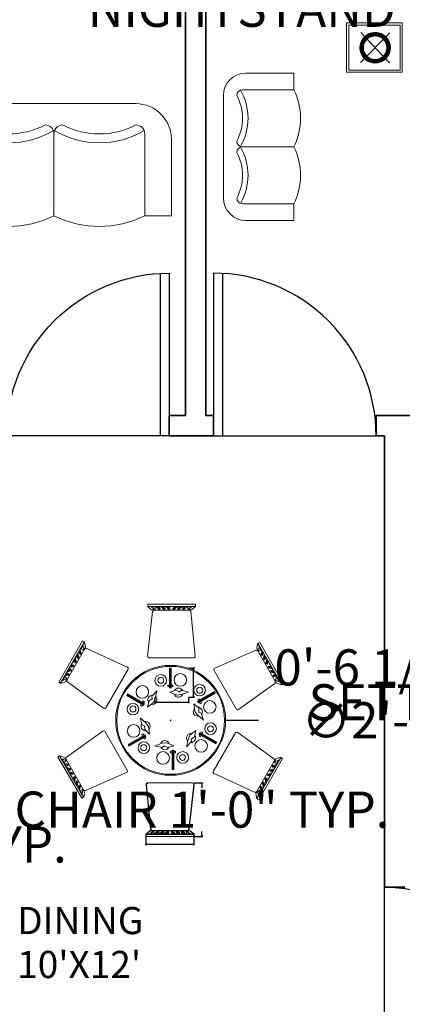
# Model space of a CAD drawing. Units: inches. Extents: x -11 to 443, y 65 to 743.
# Tile 8 of 10: x 158 to 243, y 392 to 610. Entities that reach past the tile are written whole.
import ezdxf

# ---------------------------------------------------------------- set-up
doc = ezdxf.new("R2010")
doc.units = ezdxf.units.IN
doc.header["$MEASUREMENT"] = 0
for name, color, linetype, lineweight in [('A-ANNO-DIMS', 2, 'Continuous', 18), ('A-AREA-IDEN', 2, 'Continuous', 18), ('A-DOOR', 4, 'Continuous', 25), ('A-FURN-PATT', 8, 'Continuous', 9), ('A-WALL', 7, 'Continuous', 35), ('Furniture', 7, 'Continuous', 15)]:
    doc.layers.add(name, color=color, linetype=linetype, lineweight=lineweight)
doc.styles.get("Standard").update_dxf_attribs({"font": 'italic8.shx'})
doc.dimstyles.get("Standard").update_dxf_attribs({"dimtxt": 8, "dimasz": 0.18, "dimexe": 0.18, "dimexo": 0.0625, "dimgap": 0.09, "dimtad": 0, "dimtih": 1, "dimtoh": 1, "dimzin": 0, "dimdsep": 46, "dimlunit": 3, "dimtxsty": 'Standard', "dimblk": 'CLOSEDBLANK', "dimcen": 0.09, "dimclrd": 6, "dimclre": 5, "dimclrt": 4, "dimadec": 0, "dimazin": 0, "dimtfac": 1, "dimtofl": 0, "dimtmove": 0, "dimatfit": 3, "dimfxl": 1, "dimtolj": 1, "dimtzin": 0, "dimarcsym": 0})

# ---------------------------------------------------------------- blocks, each defined once
blk = doc.blocks.new('DOOR-SWING-30')
for p, q in [((0, 30), (0, 0)), ((2, 29.93), (2, 0)), ((0, 0), (30, 0))]:
    blk.add_line(p, q)
blk.add_arc((0, 0), 30, 0, 90)
blk = doc.blocks.new('DOOR-SWING-36')
for p, q in [((36, 36), (0, 36)), ((0, 36), (0, 0)), ((35.94, 34), (0, 34))]:
    blk.add_line(p, q)
blk.add_arc((0, 36), 36, 270, 0)
blk = doc.blocks.new('NIGHTSTAND-LAMP')
for p, q in [((0, 10.9), (0, 0)), ((12.32, 10.9), (0, 10.9)), ((12.32, 0), (12.32, 10.9)), ((0.49, 10.41), (0.49, 0.49)), ((11.83, 10.41), (0.49, 10.41)), ((2.81, 2.1), (9.21, 8.77)), ((11.83, 0.49), (11.83, 10.41)), ((2.74, 8.7), (9.27, 2.17)), ((0.49, 0.49), (11.83, 0.49)), ((0, 0), (12.32, 0))]:
    blk.add_line(p, q)
for radius in [3.39, 2.6]:
    blk.add_circle((6.01, 5.43), radius)
blk = doc.blocks.new('LOVESEAT')
for p, q in [((0, 24.8, -27), (0, 7.87, -27)), ((0, 24.8, -27), (5.91, 24.8, -27)), ((5.91, 6.69, -27), (5.91, 24.8, -27)), ((25.98, 24.8, -27), (25.98, 6.69, -27)), ((25.98, 6.69, -27), (25.98, 24.8, -27)), ((46.06, 6.69, -27), (46.06, 24.8, -27)), ((46.06, 24.8, -27), (46.06, 6.69, -27)), ((46.06, 6.69, -27), (46.06, 24.8, -27)), ((51.97, 24.8, -27), (46.06, 24.8, -27)), ((51.97, 7.87, -27), (51.97, 24.8, -27)), ((7.87, 0, -27), (44.09, 0, -27))]:
    blk.add_line(p, q)
for centre, radius, start, end in [((15.94, 4.65, -27), 22.51, 63.519, 116.481), ((36.02, 4.65, -27), 22.51, 63.519, 116.481), ((7.87, 7.87, -27), 7.87, 180, 270), ((7.87, 6.69, -27), 1.97, 180, 270), ((15.94, -10.84, -27), 19.5, 59.4911, 120.5089), ((15.94, -10.84, -27), 17.53, 62.5861, 117.4139), ((24.02, 6.69, -27), 1.97, 270, 0), ((27.95, 6.69, -27), 1.97, 180, 270), ((36.02, -10.84, -27), 19.5, 59.4911, 120.5089), ((36.02, -10.84, -27), 17.53, 62.5861, 117.4139), ((44.09, 7.87, -27), 7.87, 270, 0), ((44.09, 6.69, -27), 1.97, 270, 0)]:
    blk.add_arc(centre, radius, start, end)
blk = doc.blocks.new('CHAIR-DINING')
for p, q in [((0, 11.35), (0.9, 10.62)), ((0.07, 11.85), (0.07, 11.38)), ((10.63, 11.85), (0.07, 11.85)), ((0.07, 11.38), (10.63, 11.38)), ((0.87, 11.24), (1.74, 11.27)), ((1.66, 10.66), (0.87, 11.24)), ((1.74, 11.27), (1.7, 10.77)), ((1.95, 11.31), (2.49, 10.77)), ((2.24, 11.27), (2.46, 11.27)), ((2.78, 10.77), (2.24, 11.27)), ((2.46, 11.27), (2.71, 11.06)), ((2.71, 11.06), (2.78, 11.13)), ((2.78, 11.13), (2.82, 10.8)), ((3.04, 11.31), (3.58, 10.77)), ((3.33, 11.27), (3.54, 11.27)), ((3.87, 10.77), (3.33, 11.27)), ((3.54, 11.27), (3.8, 11.06)), ((3.8, 11.06), (3.87, 11.13)), ((3.87, 11.13), (3.9, 10.8)), ((4.12, 11.31), (4.66, 10.77)), ((4.41, 11.27), (4.63, 11.27)), ((4.95, 10.77), (4.41, 11.27)), ((4.63, 11.27), (4.88, 11.06)), ((4.88, 11.06), (4.95, 11.13)), ((4.95, 11.13), (4.99, 10.8)), ((5.68, 11.13), (5.64, 10.8)), ((5.68, 10.77), (6.22, 11.27)), ((5.75, 11.06), (5.68, 11.13)), ((6, 11.27), (5.75, 11.06)), ((6.51, 11.31), (5.97, 10.77)), ((6.22, 11.27), (6, 11.27)), ((6.76, 11.13), (6.72, 10.8)), ((6.76, 10.77), (7.3, 11.27)), ((6.83, 11.06), (6.76, 11.13)), ((7.09, 11.27), (6.83, 11.06)), ((7.59, 11.31), (7.05, 10.77)), ((7.3, 11.27), (7.09, 11.27)), ((7.85, 11.13), (7.81, 10.8)), ((7.85, 10.77), (8.39, 11.27)), ((7.92, 11.06), (7.85, 11.13)), ((8.17, 11.27), (7.92, 11.06)), ((8.68, 11.31), (8.13, 10.77)), ((8.39, 11.27), (8.17, 11.27)), ((8.89, 11.27), (8.93, 10.77)), ((9.76, 11.24), (8.89, 11.27)), ((8.97, 10.66), (9.76, 11.24)), ((10.63, 11.35), (9.73, 10.62)), ((10.63, 11.38), (10.63, 11.85)), ((0.04, 0.4), (1.12, 10.23)), ((0.9, 10.62), (1.66, 10.66)), ((1.48, 10.55), (9.25, 10.55)), ((2.49, 10.77), (2.78, 10.77)), ((3.58, 10.77), (3.87, 10.77)), ((4.66, 10.77), (4.95, 10.77)), ((5.97, 10.77), (5.68, 10.77)), ((7.05, 10.77), (6.76, 10.77)), ((8.13, 10.77), (7.85, 10.77)), ((9.73, 10.62), (8.97, 10.66)), ((9.61, 10.22), (10.55, 0.4)), ((10.2, 0), (0.4, 0))]:
    blk.add_line(p, q)
for centre, start, end in [((1.48, 10.19), 90, 173.7428), ((9.25, 10.19), 5.4801, 90), ((0.4, 0.36), 173.7428, 270), ((10.2, 0.36), 270, 5.4801)]:
    blk.add_arc(centre, 0.362, start, end)
blk = doc.blocks.new('DINING-PLACE-SETTING')
for p, q in [((3.22, 6.41, 2.06), (3.22, 2.09, 2.06)), ((3.35, 6.41, 2.06), (3.22, 6.41, 2.06)), ((3.35, 2.09, 2.06), (3.35, 6.41, 2.06)), ((3.47, 6.41, 2.06), (3.47, 2.09, 2.06)), ((3.61, 6.41, 2.06), (3.47, 6.41, 2.06)), ((3.61, 2.09, 2.06), (3.61, 6.41, 2.06)), ((2.87, 2.69, 2.06), (2.87, 2.34, 2.06)), ((3.22, 2.69, 2.06), (2.87, 2.69, 2.06)), ((2.87, 2.34, 2.06), (3.22, 2.34, 2.06)), ((3.47, 2.69, 2.06), (3.35, 2.69, 2.06)), ((3.35, 2.34, 2.06), (3.47, 2.34, 2.06)), ((3.99, 2.69, 2.06), (3.61, 2.69, 2.06)), ((3.61, 2.34, 2.06), (3.99, 2.34, 2.06)), ((3.99, 2.34, 2.06), (3.99, 2.69, 2.06)), ((3.22, 2.09, 2.06), (3.35, 2.09, 2.06)), ((4.66, 1.55, 2.06), (3.27, 1.14, 2.06)), ((3.27, 1.14, 2.06), (4.83, 0.47, 2.06)), ((3.47, 2.09, 2.06), (3.61, 2.09, 2.06)), ((5.42, 1.19, 2.06), (4.66, 1.55, 2.06)), ((4.83, 0.47, 2.06), (5.82, 0.61, 2.06)), ((5.86, 1.53, 2.06), (5.42, 1.19, 2.06)), ((5.82, 0.61, 2.06), (7.45, 1.14, 2.06)), ((7.45, 1.14, 2.06), (5.86, 1.53, 2.06))]:
    blk.add_line(p, q)
for centre, radius in [((1.29, 3.72, 2.06), 1.29), ((1.32, 3.74, 2.06), 0.665), ((5.63, 3.83, 2.06), 1.39)]:
    blk.add_circle(centre, radius)
for start, end in [(197.0611, 344.0662), (26.6641, 154.1442)]:
    blk.add_arc((5.23, 1.01, 2.06), 1.01, start, end)
blk = doc.blocks.new('_ClosedBlank')
at = {"color": 0, "linetype": 'ByBlock', "lineweight": -2}
for p, q in [((-1, 0.167), (0, 0)), ((-1, 0.167), (-1, -0.167)), ((0, 0), (-1, -0.167))]:
    blk.add_line(p, q, dxfattribs=at)
blk = doc.blocks.new('*D26')
at = {"layer": 'A-ANNO-DIMS', "color": 5, "lineweight": -2, "transparency": 16777216}
for p, q in [((133.01, 610.6), (133.01, 612.57)), ((145.34, 610.6), (145.34, 612.57))]:
    blk.add_line(p, q, dxfattribs=at)
at = {"layer": 'A-ANNO-DIMS', "color": 6, "lineweight": -2, "transparency": 16777216}
for p, q in [((133.19, 612.39), (145.16, 612.39)), ((145.34, 612.39), (145.52, 612.39))]:
    blk.add_line(p, q, dxfattribs=at)
at = {"layer": 'Defpoints', "color": 0, "lineweight": 100, "transparency": 16777216}
for p in [(145.34, 612.39), (133.01, 610.54), (145.34, 610.54)]:
    blk.add_point(p, dxfattribs=at)
at = {"layer": 'A-ANNO-DIMS', "color": 6, "lineweight": -2, "transparency": 16777216, "xscale": 0.18, "yscale": 0.18, "zscale": 0.18, "rotation": 180}
blk.add_blockref('_ClosedBlank', (133.01, 612.39), dxfattribs=at)
at = {"layer": 'A-ANNO-DIMS', "color": 6, "lineweight": -2, "transparency": 16777216, "xscale": 0.18, "yscale": 0.18, "zscale": 0.18}
blk.add_blockref('_ClosedBlank', (145.34, 612.39), dxfattribs=at)
at = {"layer": 'A-ANNO-DIMS', "color": 4, "transparency": 16777216, "insert": (242.18, 612.39), "char_height": 8, "attachment_point": 5}
blk.add_mtext('\\A1;NIGHTSTAND 1\'-0 1/2" TYP.', dxfattribs=at)
blk = doc.blocks.new('*D28')
at = {"layer": 'A-ANNO-DIMS', "color": 5, "lineweight": -2, "transparency": 16777216}
for p, q in [((196.6, 441.21), (198.5, 441.21)), ((196.6, 429.36), (198.5, 429.36))]:
    blk.add_line(p, q, dxfattribs=at)
at = {"layer": 'A-ANNO-DIMS', "color": 6, "lineweight": -2, "transparency": 16777216}
for p, q in [((198.32, 441.03), (198.32, 440.14)), ((198.32, 429.54), (198.32, 430.44))]:
    blk.add_line(p, q, dxfattribs=at)
at = {"layer": 'Defpoints', "color": 0, "lineweight": 100, "transparency": 16777216}
for p in [(196.54, 441.21), (196.54, 429.36), (198.32, 429.36)]:
    blk.add_point(p, dxfattribs=at)
at = {"layer": 'A-ANNO-DIMS', "color": 6, "lineweight": -2, "transparency": 16777216, "xscale": 0.18, "yscale": 0.18, "zscale": 0.18}
for p, rotation in [((198.32, 441.21), 90), ((198.32, 429.36), 270)]:
    blk.add_blockref('_ClosedBlank', p, dxfattribs=dict(at, rotation=rotation))
at = {"layer": 'A-ANNO-DIMS', "color": 4, "transparency": 16777216, "insert": (198.32, 435.29), "char_height": 8, "attachment_point": 5}
blk.add_mtext('\\A1;CHAIR 1\'-0" TYP.', dxfattribs=at)
blk = doc.blocks.new('*D29')
at = {"layer": 'A-ANNO-DIMS', "color": 5, "lineweight": -2, "transparency": 16777216}
for p, q in [((185.91, 429.3), (185.91, 427.4)), ((196.54, 429.3), (196.54, 427.4))]:
    blk.add_line(p, q, dxfattribs=at)
at = {"layer": 'A-ANNO-DIMS', "color": 6, "lineweight": -2, "transparency": 16777216}
for p, q in [((185.91, 427.58), (185.73, 427.58)), ((196.36, 427.58), (186.09, 427.58))]:
    blk.add_line(p, q, dxfattribs=at)
at = {"layer": 'Defpoints', "color": 0, "lineweight": 100, "transparency": 16777216}
for p in [(185.91, 429.36), (196.54, 429.36), (185.91, 427.58)]:
    blk.add_point(p, dxfattribs=at)
at = {"layer": 'A-ANNO-DIMS', "color": 6, "lineweight": -2, "transparency": 16777216, "xscale": 0.18, "yscale": 0.18, "zscale": 0.18, "rotation": 180}
blk.add_blockref('_ClosedBlank', (185.91, 427.58), dxfattribs=at)
at = {"layer": 'A-ANNO-DIMS', "color": 6, "lineweight": -2, "transparency": 16777216, "xscale": 0.18, "yscale": 0.18, "zscale": 0.18}
blk.add_blockref('_ClosedBlank', (196.54, 427.58), dxfattribs=at)
at = {"layer": 'A-ANNO-DIMS', "color": 4, "transparency": 16777216, "insert": (131.55, 427.58), "char_height": 8, "attachment_point": 5}
blk.add_mtext('\\A1;0\'-10 1/2" TYP.', dxfattribs=at)
blk = doc.blocks.new('*D30')
at = {"layer": 'A-ANNO-DIMS', "color": 5, "lineweight": -2, "transparency": 16777216}
for p, q in [((187.91, 460.07), (187.91, 458.84)), ((195.36, 460.07), (195.36, 458.84))]:
    blk.add_line(p, q, dxfattribs=at)
at = {"layer": 'A-ANNO-DIMS', "color": 6, "lineweight": -2, "transparency": 16777216}
for p, q in [((188.09, 459.02), (195.18, 459.02)), ((195.36, 459.02), (195.54, 459.02))]:
    blk.add_line(p, q, dxfattribs=at)
at = {"layer": 'Defpoints', "color": 0, "lineweight": 100, "transparency": 16777216}
for p in [(187.91, 460.14), (195.36, 460.14), (195.36, 459.02)]:
    blk.add_point(p, dxfattribs=at)
at = {"layer": 'A-ANNO-DIMS', "color": 6, "lineweight": -2, "transparency": 16777216, "xscale": 0.18, "yscale": 0.18, "zscale": 0.18, "rotation": 180}
blk.add_blockref('_ClosedBlank', (187.91, 459.02), dxfattribs=at)
at = {"layer": 'A-ANNO-DIMS', "color": 6, "lineweight": -2, "transparency": 16777216, "xscale": 0.18, "yscale": 0.18, "zscale": 0.18}
blk.add_blockref('_ClosedBlank', (195.36, 459.02), dxfattribs=at)
at = {"layer": 'A-ANNO-DIMS', "color": 4, "transparency": 16777216, "insert": (279.25, 459.02), "char_height": 8, "attachment_point": 5}
blk.add_mtext('\\A1;SETTING 0\'-7 1/2" TYP.', dxfattribs=at)
blk = doc.blocks.new('*D31')
at = {"layer": 'A-ANNO-DIMS', "color": 5, "lineweight": -2, "transparency": 16777216}
for p, q in [((195.43, 466.55), (196.66, 466.55)), ((195.43, 460.14), (196.66, 460.14))]:
    blk.add_line(p, q, dxfattribs=at)
at = {"layer": 'A-ANNO-DIMS', "color": 6, "lineweight": -2, "transparency": 16777216}
for p, q in [((196.48, 466.55), (196.48, 466.73)), ((196.48, 466.73), (196.66, 466.73)), ((196.48, 460.32), (196.48, 466.37))]:
    blk.add_line(p, q, dxfattribs=at)
at = {"layer": 'Defpoints', "color": 0, "lineweight": 100, "transparency": 16777216}
for p in [(195.36, 466.55), (196.48, 466.55), (195.36, 460.14)]:
    blk.add_point(p, dxfattribs=at)
at = {"layer": 'A-ANNO-DIMS', "color": 6, "lineweight": -2, "transparency": 16777216, "xscale": 0.18, "yscale": 0.18, "zscale": 0.18}
for p, rotation in [((196.48, 466.55), 90), ((196.48, 460.14), 270)]:
    blk.add_blockref('_ClosedBlank', p, dxfattribs=dict(at, rotation=rotation))
at = {"layer": 'A-ANNO-DIMS', "color": 4, "transparency": 16777216, "insert": (248.18, 466.73), "char_height": 8, "attachment_point": 5}
blk.add_mtext('\\A1;0\'-6 1/2" TYP.', dxfattribs=at)
blk = doc.blocks.new('*D41')
at = {"layer": 'A-ANNO-DIMS', "color": 5, "lineweight": -2, "transparency": 16777216}
for p, q in [((191.4, 454.94), (191.4, 455.12)), ((191.31, 455.03), (191.49, 455.03))]:
    blk.add_line(p, q, dxfattribs=at)
at = {"layer": 'A-ANNO-DIMS', "color": 6, "lineweight": -2, "transparency": 16777216}
blk.add_line((210.85, 455.03), (203.74, 455.03), dxfattribs=at)
at = {"layer": 'Defpoints', "color": 0, "lineweight": 100, "transparency": 16777216}
for p in [(179.23, 455.03), (203.56, 455.03)]:
    blk.add_point(p, dxfattribs=at)
at = {"layer": 'A-ANNO-DIMS', "color": 6, "lineweight": -2, "transparency": 16777216, "xscale": 0.18, "yscale": 0.18, "zscale": 0.18, "rotation": 179.9993686908669}
blk.add_blockref('_ClosedBlank', (203.56, 455.03), dxfattribs=at)
at = {"layer": 'A-ANNO-DIMS', "color": 4, "transparency": 16777216, "insert": (247.32, 455.03), "char_height": 8, "attachment_point": 5}
blk.add_mtext('\\A1;∅2\'-0 1/2"', dxfattribs=at)

msp = doc.modelspace()

# ---------------------------------------------------------------- hatches: boundary and pattern name
at = {"layer": 'A-FURN-PATT'}
h = msp.add_hatch(dxfattribs=at)
h.set_pattern_fill('ANSI37', color=256, scale=0.6260848, angle=45, style=0)
h.paths.add_polyline_path([(240.028, 603.779), (240.026, 603.912), (240.018, 604.045), (240.005, 604.177), (239.987, 604.309), (239.963, 604.44), (239.935, 604.57), (239.901, 604.698), (239.863, 604.826), (239.819, 604.951), (239.771, 605.075), (239.717, 605.197), (239.659, 605.317), (239.596, 605.434), (239.529, 605.549), (239.457, 605.661), (239.381, 605.77), (239.301, 605.876), (239.217, 605.979), (239.128, 606.079), (239.036, 606.175), (238.94, 606.267), (238.841, 606.355), (238.738, 606.44), (238.632, 606.52), (238.523, 606.596), (238.411, 606.668), (238.296, 606.735), (238.178, 606.798), (238.059, 606.856), (237.937, 606.909), (237.813, 606.958), (237.687, 607.001), (237.56, 607.04), (237.431, 607.073), (237.301, 607.102), (237.17, 607.125), (237.038, 607.144), (236.906, 607.157), (236.773, 607.164), (236.64, 607.167), (236.507, 607.164), (236.374, 607.157), (236.242, 607.144), (236.11, 607.125), (235.979, 607.102), (235.849, 607.073), (235.72, 607.04), (235.593, 607.001), (235.467, 606.958), (235.344, 606.909), (235.222, 606.856), (235.102, 606.798), (234.985, 606.735), (234.87, 606.668), (234.758, 606.596), (234.649, 606.52), (234.543, 606.44), (234.44, 606.355), (234.34, 606.267), (234.244, 606.175), (234.152, 606.079), (234.064, 605.979), (233.979, 605.876), (233.899, 605.77), (233.823, 605.661), (233.751, 605.549), (233.684, 605.434), (233.621, 605.317), (233.563, 605.197), (233.51, 605.075), (233.461, 604.951), (233.418, 604.826), (233.379, 604.698), (233.346, 604.57), (233.317, 604.44), (233.294, 604.309), (233.275, 604.177), (233.262, 604.045), (233.255, 603.912), (233.252, 603.779), (233.255, 603.646), (233.262, 603.513), (233.275, 603.38), (233.294, 603.249), (233.317, 603.118), (233.346, 602.988), (233.379, 602.859), (233.418, 602.732), (233.461, 602.606), (233.51, 602.482), (233.563, 602.36), (233.621, 602.24), (233.684, 602.123), (233.751, 602.008), (233.823, 601.896), (233.899, 601.787), (233.979, 601.681), (234.064, 601.578), (234.152, 601.479), (234.244, 601.383), (234.34, 601.291), (234.44, 601.202), (234.543, 601.118), (234.649, 601.038), (234.758, 600.961), (234.87, 600.89), (234.985, 600.822), (235.102, 600.76), (235.222, 600.702), (235.344, 600.648), (235.467, 600.6), (235.593, 600.556), (235.72, 600.518), (235.849, 600.484), (235.979, 600.456), (236.11, 600.432), (236.242, 600.414), (236.374, 600.401), (236.507, 600.393), (236.64, 600.39), (236.773, 600.393), (236.906, 600.401), (237.038, 600.414), (237.17, 600.432), (237.301, 600.456), (237.431, 600.484), (237.56, 600.518), (237.687, 600.556), (237.813, 600.6), (237.937, 600.648), (238.059, 600.702), (238.178, 600.76), (238.296, 600.822), (238.411, 600.89), (238.523, 600.961), (238.632, 601.038), (238.738, 601.118), (238.841, 601.202), (238.94, 601.291), (239.036, 601.383), (239.128, 601.479), (239.217, 601.578), (239.301, 601.681), (239.381, 601.787), (239.457, 601.896), (239.529, 602.008), (239.596, 602.123), (239.659, 602.24), (239.717, 602.36), (239.771, 602.482), (239.819, 602.606), (239.863, 602.732), (239.901, 602.859), (239.935, 602.988), (239.963, 603.118), (239.987, 603.249), (240.005, 603.38), (240.018, 603.513), (240.026, 603.646)])
h.paths.add_polyline_path([(239.245, 603.779), (239.243, 603.676), (239.237, 603.574), (239.227, 603.473), (239.213, 603.371), (239.195, 603.271), (239.173, 603.171), (239.147, 603.072), (239.118, 602.974), (239.084, 602.877), (239.047, 602.782), (239.006, 602.688), (238.961, 602.596), (238.913, 602.506), (238.861, 602.418), (238.806, 602.332), (238.748, 602.248), (238.686, 602.166), (238.621, 602.087), (238.553, 602.011), (238.482, 601.937), (238.408, 601.866), (238.332, 601.798), (238.253, 601.733), (238.171, 601.671), (238.087, 601.613), (238.001, 601.558), (237.913, 601.506), (237.823, 601.458), (237.731, 601.413), (237.637, 601.372), (237.542, 601.335), (237.445, 601.301), (237.347, 601.272), (237.248, 601.246), (237.148, 601.224), (237.048, 601.206), (236.946, 601.192), (236.845, 601.182), (236.742, 601.176), (236.64, 601.174), (236.538, 601.176), (236.436, 601.182), (236.334, 601.192), (236.233, 601.206), (236.132, 601.224), (236.032, 601.246), (235.933, 601.272), (235.835, 601.301), (235.739, 601.335), (235.643, 601.372), (235.55, 601.413), (235.458, 601.458), (235.367, 601.506), (235.279, 601.558), (235.193, 601.613), (235.109, 601.671), (235.028, 601.733), (234.949, 601.798), (234.872, 601.866), (234.798, 601.937), (234.727, 602.011), (234.659, 602.087), (234.595, 602.166), (234.533, 602.248), (234.474, 602.332), (234.419, 602.418), (234.368, 602.506), (234.319, 602.596), (234.275, 602.688), (234.234, 602.782), (234.196, 602.877), (234.163, 602.974), (234.133, 603.072), (234.107, 603.171), (234.085, 603.271), (234.067, 603.371), (234.053, 603.473), (234.043, 603.574), (234.037, 603.676), (234.035, 603.779), (234.037, 603.881), (234.043, 603.983), (234.053, 604.085), (234.067, 604.186), (234.085, 604.287), (234.107, 604.387), (234.133, 604.486), (234.163, 604.584), (234.196, 604.68), (234.234, 604.776), (234.275, 604.869), (234.319, 604.961), (234.368, 605.051), (234.419, 605.14), (234.474, 605.226), (234.533, 605.31), (234.595, 605.391), (234.659, 605.47), (234.727, 605.547), (234.798, 605.621), (234.872, 605.691), (234.949, 605.759), (235.028, 605.824), (235.109, 605.886), (235.193, 605.945), (235.279, 606), (235.367, 606.051), (235.458, 606.1), (235.55, 606.144), (235.643, 606.185), (235.739, 606.223), (235.835, 606.256), (235.933, 606.286), (236.032, 606.312), (236.132, 606.333), (236.233, 606.351), (236.334, 606.365), (236.436, 606.376), (236.538, 606.382), (236.64, 606.384), (236.742, 606.382), (236.845, 606.376), (236.946, 606.365), (237.048, 606.351), (237.148, 606.333), (237.248, 606.312), (237.347, 606.286), (237.445, 606.256), (237.542, 606.223), (237.637, 606.185), (237.731, 606.144), (237.823, 606.1), (237.913, 606.051), (238.001, 606), (238.087, 605.945), (238.171, 605.886), (238.253, 605.824), (238.332, 605.759), (238.408, 605.691), (238.482, 605.621), (238.553, 605.547), (238.621, 605.47), (238.686, 605.391), (238.748, 605.31), (238.806, 605.226), (238.861, 605.14), (238.913, 605.051), (238.961, 604.961), (239.006, 604.869), (239.047, 604.776), (239.084, 604.68), (239.118, 604.584), (239.147, 604.486), (239.173, 604.387), (239.195, 604.287), (239.213, 604.186), (239.227, 604.085), (239.237, 603.983), (239.243, 603.881)], flags=0)

# ---------------------------------------------------------------- linework, layer by layer
at = {"layer": 'A-WALL'}
for p, q in [((194.709, 616.92), (194.709, 522.42)), ((199.209, 616.92), (199.209, 522.42)), ((191.085, 522.42), (191.085, 517.92)), ((191.085, 522.42), (194.709, 522.42)), ((199.209, 522.42), (200.859, 522.42)), ((200.859, 517.92), (200.859, 522.42)), ((236.859, 517.92), (236.859, 522.42)), ((236.859, 522.42), (323.209, 522.42)), ((191.085, 517.92), (200.859, 517.92)), ((236.859, 517.92), (238.709, 517.92)), ((238.709, 418.17), (238.709, 517.92)), ((243.209, 418.17), (238.709, 418.17))]:
    msp.add_line(p, q, dxfattribs=at)
at = {"layer": 'Furniture'}
for p, q in [((218.649, 598.186), (208.023, 598.186)), ((218.649, 598.186), (218.649, 594.479)), ((207.282, 594.479), (218.649, 594.479)), ((203.081, 593.244), (203.081, 570.51)), ((218.649, 581.877), (207.282, 581.877)), ((207.282, 581.877), (218.649, 581.877)), ((207.282, 569.275), (218.649, 569.275)), ((218.649, 569.275), (207.282, 569.275)), ((207.282, 569.275), (218.649, 569.275)), ((218.649, 565.568), (218.649, 569.275)), ((208.023, 565.568), (218.649, 565.568))]:
    msp.add_line(p, q, dxfattribs=at)
for radius in [12.161, 11.935]:
    msp.add_circle((191.395, 455.031), radius, dxfattribs=at)
for centre, radius, start, end in [((208.023, 593.244), 4.942, 90, 180), ((207.282, 593.244), 1.236, 90, 180), ((206, 588.178), 14.131, 333.51896, 26.48104), ((196.279, 588.178), 11.002, 332.58608, 27.41392), ((196.279, 588.178), 12.238, 329.49109, 30.50891), ((207.282, 583.113), 1.236, 180, 270), ((207.282, 580.642), 1.236, 90, 180), ((196.279, 575.576), 12.238, 329.49109, 30.50891), ((206, 575.576), 14.131, 333.51896, 26.48104), ((196.279, 575.576), 11.002, 332.58608, 27.41392), ((208.023, 570.51), 4.942, 180, 270), ((207.282, 570.51), 1.236, 180, 270)]:
    msp.add_arc(centre, radius, start, end, dxfattribs=at)

# ---------------------------------------------------------------- block references
at = {"layer": 'A-DOOR', "extrusion": (0, 0, -1), "zscale": -1}
for name, p, rotation in [('DOOR-SWING-36', (-155.086, 517.92), 90.00000000000014), ('DOOR-SWING-30', (-238.709, 388.169), 90.00000000000003)]:
    msp.add_blockref(name, p, dxfattribs=dict(at, rotation=rotation))
at = {"layer": 'A-DOOR', "rotation": 90.0000000000001}
msp.add_blockref('DOOR-SWING-36', (236.859, 517.92), dxfattribs=at)
at = {"layer": 'Furniture', "extrusion": (0, 0, -1), "zscale": -1}
msp.add_blockref('NIGHTSTAND-LAMP', (-242.647, 598.345), dxfattribs=at)
at = {"layer": 'Furniture'}
for name, p, rotation in [('LOVESEAT', (191.555, 591.409), 180), ('CHAIR-DINING', (176.857, 457.484), 59.99999999999355), ('CHAIR-DINING', (200.789, 466.395), 300.0000000000028), ('DINING-PLACE-SETTING', (185.618, 454.528), 60.00000000001144), ('DINING-PLACE-SETTING', (193.92, 460.961), 300.0000000000051), ('DINING-PLACE-SETTING', (189.332, 449.735), 120.0000000000119), ('DINING-PLACE-SETTING', (197.634, 456.168), 240.0000000000069), ('CHAIR-DINING', (182.002, 443.668), 120.0000000000038), ('CHAIR-DINING', (205.933, 452.578), 240.0000000000063), ('DINING-PLACE-SETTING', (195.34, 450.555), 180), ('CHAIR-DINING', (196.54, 441.214), 180), ('CHAIR-DINING', (196.633, 441.18), 180)]:
    msp.add_blockref(name, p, dxfattribs=dict(at, rotation=rotation))
for name, p in [('CHAIR-DINING', (186.251, 468.848)), ('DINING-PLACE-SETTING', (187.912, 460.141))]:
    msp.add_blockref(name, p, dxfattribs=at)

# ---------------------------------------------------------------- texts
at = {"layer": 'A-AREA-IDEN'}
for s, p in [('DINING', (157.447, 407.752)), ("10'X12'", (157.447, 398.038))]:
    msp.add_text(s, height=6, dxfattribs=at).set_placement(p)

# ---------------------------------------------------------------- dimensions: what is measured, and where the dimension line sits
at = {"layer": 'A-ANNO-DIMS'}
for base, p1, p2, text, picture, middle in [((145.337, 612.387), (133.013, 610.539), (145.337, 610.539), 'NIGHTSTAND <> TYP.', '*D26', (242.179, 612.387)), ((195.365, 459.019), (187.912, 460.137), (195.365, 460.137), 'SETTING <> TYP.', '*D30', (279.254, 459.019))]:
    dim = msp.add_linear_dim(base=base, p1=p1, p2=p2, text=text, dimstyle='Standard', override={"dimdec": 1, "dimlfac": 1, "dimrnd": 0, "dimzin": 1, "dimdsep": 46, "dimlunit": 4, "dimfrac": 2}, dxfattribs=at)
    dim.commit()
    dim.dimension.update_dxf_attribs({"geometry": picture, "text_midpoint": middle})
for base, p1, p2, angle, text, picture, middle in [((196.483, 466.551), (195.365, 460.137), (195.365, 466.551), 90, '<> TYP.', '*D31', (248.181, 466.731)), ((198.318, 429.362), (196.54, 441.214), (196.54, 429.362), 270, 'CHAIR <> TYP.', '*D28', (198.318, 435.288)), ((185.911, 427.584), (196.54, 429.362), (185.911, 429.362), 180, '<> TYP.', '*D29', (131.545, 427.584))]:
    dim = msp.add_linear_dim(base=base, p1=p1, p2=p2, angle=angle, text=text, dimstyle='Standard', override={"dimdec": 1, "dimlfac": 1, "dimrnd": 0, "dimzin": 1, "dimdsep": 46, "dimlunit": 4, "dimfrac": 2}, dxfattribs=at)
    dim.commit()
    dim.dimension.update_dxf_attribs({"geometry": picture, "text_midpoint": middle})
dim = msp.add_diameter_dim_2p(p1=(179.234, 455.031), p2=(203.557, 455.031), dimstyle='Standard', override={"dimdec": 1, "dimlfac": 1, "dimrnd": 0, "dimzin": 1, "dimdsep": 46, "dimlunit": 4, "dimfrac": 2}, dxfattribs=at)
dim.commit()
dim.dimension.update_dxf_attribs({"geometry": '*D41', "text_midpoint": (210.854, 455.031), "dimtype": 163})

doc.saveas('drawing.dxf')
